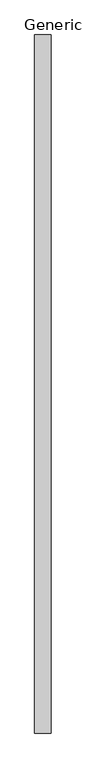
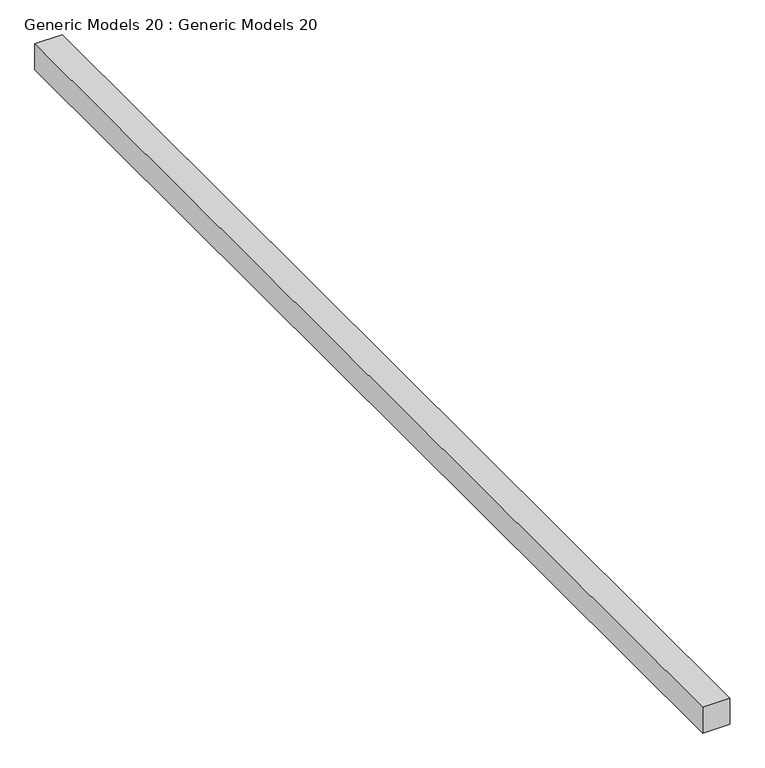
"""IFC4 building model written with IfcOpenShell, lengths in millimetres: proxy geometry, Generic Models 20 : Generic Models 20."""

from ifc_helpers import new_model, si_unit, frame, origin, place, context, project, spatial, polyline, outline, extrude, source, transform, mapped, element, save


def generic_models_20_generic_models_20_2b057986(model_context):
    return source(origin(), model_context, "Body", "SweptSolid", [
        extrude(outline(polyline([(-15581.438074, -5966.8213044), (-15581.438074, 6948.1514639), (-15276.638074, 6948.1514639), (-15276.638074, -5966.8213044), (-15581.438074, -5966.8213044)])), frame((0.0, 0.0, 12801.6), z_axis=(0.0, 0.0, 1.0), x_axis=(1.0, 0.0, 0.0)), (0.0, 0.0, 1.0), 304.8),
    ])


if __name__ == "__main__":
    model = new_model("IFC4")
    model_context = context("Model", 3, world=origin())
    ifc_project = project(units=[si_unit("LENGTHUNIT", "METRE", prefix="MILLI")], contexts=[model_context])
    site = spatial("IfcSite", under=ifc_project)
    building = spatial("IfcBuilding", under=site)
    placement = place(None, origin())
    generic_models_20_generic_models_20_shape = generic_models_20_generic_models_20_2b057986(model_context)
    element("IfcBuildingElementProxy", 1, Name="Generic Models 20 : Generic Models 20", ObjectType="Generic Models 20 : Generic Models 20", at=placement, inside=building, context=model_context, shape_type="MappedRepresentation", body=[
        mapped(generic_models_20_generic_models_20_shape, transform((0.0, 0.0, 0.0), x_axis=(1.0, 0.0, 0.0), y_axis=(0.0, 1.0, 0.0), z_axis=(0.0, 0.0, 1.0))),
    ])
    save(model, "model.ifc")
